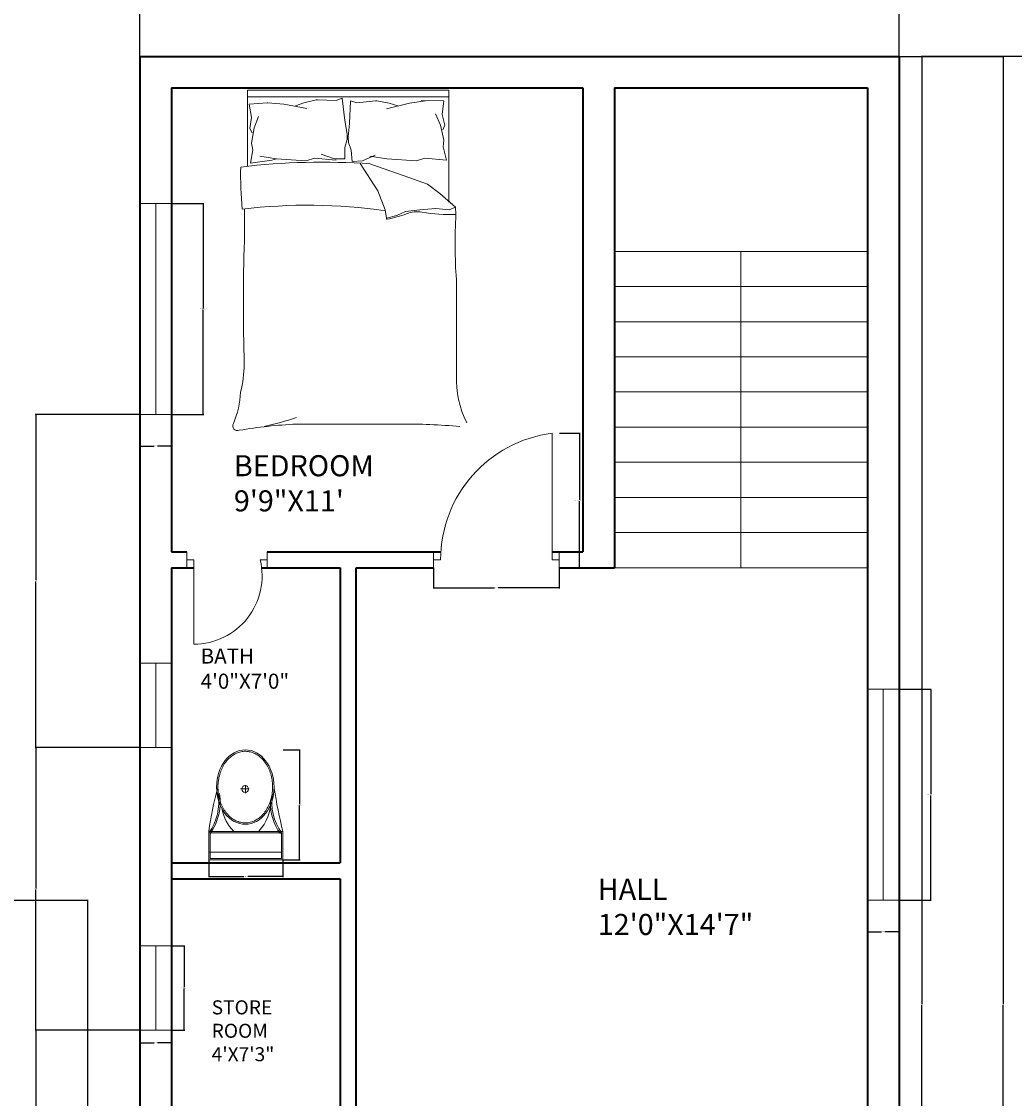
# Model space of a CAD drawing. Units: inches. Extents: x 2003 to 3241, y 1726 to 2849.
# Tile 4 of 7: x 2317 to 2599, y 2073 to 2380. Entities that reach past the tile are written whole.
import ezdxf

# ---------------------------------------------------------------- set-up
doc = ezdxf.new("R2010")
doc.units = ezdxf.units.IN
for name, color, linetype, lineweight in [('A-ANNO-DIMS', 2, 'Continuous', 18), ('A-AREA-IDEN', 7, 'Continuous', 18), ('A-DOOR', 3, 'Continuous', 18), ('A-FLOR-FIXT', 9, 'Continuous', 18), ('A-FLOR-STRS', 7, 'Continuous', 18), ('A-FURN', 8, 'Continuous', 13), ('A-GLAZ', 4, 'Continuous', 18), ('A-WALL', 7, 'Continuous', 35)]:
    doc.layers.add(name, color=color, linetype=linetype, lineweight=lineweight)
doc.styles.add('Annotative', font='arial.ttf')
doc.styles.get("Standard").update_dxf_attribs({"font": 'arial.ttf'})
doc.dimstyles.get("Standard").update_dxf_attribs({"dimtxt": 0.18, "dimasz": 0.18, "dimexe": 0.18, "dimexo": 0.0625, "dimgap": 0.09, "dimtad": 0, "dimtih": 1, "dimtoh": 1, "dimdec": 4, "dimzin": 0, "dimdsep": 46, "dimtxsty": 'Standard', "dimcen": 0.09, "dimadec": 0, "dimazin": 0, "dimtfac": 1, "dimtdec": 4, "dimtofl": 0, "dimtmove": 0, "dimatfit": 3, "dimfxl": 1, "dimtolj": 1, "dimtzin": 0, "dimarcsym": 0})

# ---------------------------------------------------------------- blocks, each defined once
blk = doc.blocks.new('A$C31115884')
for p, q in [((283.1, 497.7), (223.4, 497.7)), ((257.5, 466.4), (257.5, 523.2)), ((0, 200), (0, 0)), ((520, 200), (0, 200)), ((10, 190), (10, 10)), ((510, 190), (10, 190)), ((510, 10), (510, 190)), ((520, 0), (520, 200)), ((510, 54.5), (0, 54.5)), ((10, 10), (510, 10)), ((0, 0), (520, 0))]:
    blk.add_line(p, q)
blk.add_circle((255.6, 496.4), 23.6)
for centre, radius, start, end in [((2777.7, -204.6), 2807, 165.4549, 171.71327), ((-294.5, 403.3), 364.7, 324.20913, 9.34987), ((-294.5, 403.3), 374.7, 324.20913, 9.34987), ((805.8, 403.3), 364.7, 170.65013, 215.79087), ((3237, 905), 2807, 188.28673, 194.5451), ((139.5, 406.2), 293.5, 315.84364, 2.65635), ((805.8, 403.3), 374.7, 179.20365, 215.79087), ((383.6, 406.2), 293.5, 190.27735, 224.15636)]:
    blk.add_arc(centre, radius, start, end)
blk.add_ellipse((256.2, 509.9), major_axis=(0, -260.7), ratio=0.772727)
blk.add_open_spline([(256.2, 259.2), (263.1, 259.2), (270, 259.7), (287.8, 262.3), (298.7, 265.1), (319.9, 273.1), (330.2, 278.4), (350.1, 291.1), (359.7, 298.7), (377.7, 315.9), (386.2, 325.5), (401.7, 346.6), (408.8, 358.1), (421.3, 382.5), (426.8, 395.5), (435.9, 422.4), (439.5, 436.4), (444.8, 465.1), (446.5, 479.7), (447.9, 509.2), (447.6, 524), (445, 553.3), (442.7, 567.8), (436.3, 596), (432.1, 609.7), (421.9, 636), (416, 648.6), (402.5, 672.1), (395, 683), (378.6, 703), (369.8, 712.1), (351.1, 728), (341.3, 734.8), (320.9, 746.2), (310.4, 750.7), (288.9, 757.3), (278, 759.4), (256, 761), (245, 760.6), (223.1, 757.2), (212.3, 754.3), (191.1, 746.1), (180.8, 740.7), (160.9, 727.8), (151.4, 720.1), (133.5, 702.7), (125.1, 693), (109.6, 671.7), (102.6, 660.2), (90.2, 635.7), (84.9, 622.7), (76, 595.6), (72.4, 581.6), (67.2, 552.9), (65.6, 538.2), (64.4, 508.8), (64.8, 494), (67.5, 464.7), (69.9, 450.2), (76.6, 422), (80.8, 408.3), (91.1, 382.2), (97.2, 369.7), (110.8, 346.3), (118.4, 335.4), (134.8, 315.6), (143.7, 306.7), (162.4, 290.9), (172.3, 284.2), (192.8, 273), (203.3, 268.6), (224.8, 262.2), (235.8, 260.2), (249.9, 259.3), (253, 259.2), (256.2, 259.2)], degree=3, knots=[0, 0, 0, 0, 0.110105, 0.110105, 0.285049, 0.285049, 0.459994, 0.459994, 0.634938, 0.634938, 0.809882, 0.809882, 0.984827, 0.984827, 1.159771, 1.159771, 1.334715, 1.334715, 1.50966, 1.50966, 1.684604, 1.684604, 1.859549, 1.859549, 2.034493, 2.034493, 2.209437, 2.209437, 2.384382, 2.384382, 2.559326, 2.559326, 2.73427, 2.73427, 2.909215, 2.909215, 3.084159, 3.084159, 3.259103, 3.259103, 3.434048, 3.434048, 3.608992, 3.608992, 3.783936, 3.783936, 3.958881, 3.958881, 4.133825, 4.133825, 4.30877, 4.30877, 4.483714, 4.483714, 4.658658, 4.658658, 4.833603, 4.833603, 5.008547, 5.008547, 5.183491, 5.183491, 5.358436, 5.358436, 5.53338, 5.53338, 5.708324, 5.708324, 5.883269, 5.883269, 6.058213, 6.058213, 6.233158, 6.233158, 6.283185, 6.283185, 6.283185, 6.283185])
blk = doc.blocks.new('WIN-60-1')
for p, q in [((0, 60), (9, 60)), ((9, 60), (4.5, 60)), ((4.5, 60), (4.5, 0)), ((4.5, 0), (0, 0)), ((0, 0), (9, 0))]:
    blk.add_line(p, q)
blk = doc.blocks.new('WIN-60-2')
for p, q in [((9, 60), (0, 60)), ((0, 60), (4.5, 60)), ((4.5, 60), (4.5, 0)), ((4.5, 0), (0, 0)), ((0, 0), (9, 0))]:
    blk.add_line(p, q)
blk = doc.blocks.new('WIN-24-1')
for p, q in [((0, 24), (9, 24)), ((9, 24), (4.5, 24)), ((4.5, 24), (4.5, 0)), ((4.5, 0), (0, 0)), ((0, 0), (9, 0))]:
    blk.add_line(p, q)
blk = doc.blocks.new('WIN-24-2')
for p, q in [((0, 24), (9, 24)), ((9, 24), (4.5, 24)), ((4.5, 24), (4.5, 0)), ((9, 0), (0, 0)), ((4.5, 0), (9, 0))]:
    blk.add_line(p, q)
blk = doc.blocks.new('DOOR-BEDROOM-UPPER')
for p, q in [((33.76, 2.25), (33.76, 38.25)), ((0, 4.5), (0, 0)), ((35.76, 4.5), (35.76, 0)), ((0, 0), (0, 2.25)), ((0, 2.25), (2, 2.25)), ((35.76, 2.25), (33.76, 2.25)), ((35.76, 0), (35.76, 2.25))]:
    blk.add_line(p, q)
blk.add_arc((38.28, 2.25), 36.28, 97.1626, 180)
blk = doc.blocks.new('STAIR-UPPER-RUN')
for p, q in [((0, 90), (72, 90)), ((36, 0), (36, 90)), ((72, 90), (36, 90)), ((0, 80), (72, 80)), ((72, 80), (36, 80)), ((0, 70), (72, 70)), ((72, 70), (36, 70)), ((0, 60), (72, 60)), ((72, 60), (36, 60)), ((0, 50), (72, 50)), ((72, 50), (36, 50)), ((0, 40), (72, 40)), ((72, 40), (36, 40)), ((0, 30), (72, 30)), ((72, 30), (36, 30)), ((0, 20), (72, 20)), ((72, 20), (36, 20)), ((0, 10), (72, 10)), ((72, 10), (36, 10)), ((0, 0), (72, 0)), ((72, 0), (36, 0))]:
    blk.add_line(p, q)
blk = doc.blocks.new('BED-DOUBLE')
for p, q in [((4.17, 75.16), (4.17, 96.87)), ((4.17, 96.87), (61.46, 96.87)), ((4.17, 95.03), (61.46, 95.03)), ((61.46, 96.87), (61.46, 64.97)), ((4.67, 92.87), (9.81, 93.27)), ((4.67, 92.9), (5.36, 89.08)), ((9.81, 93.27), (9.93, 93.24)), ((9.93, 93.24), (14.52, 92.9)), ((14.52, 92.9), (21.1, 91.68)), ((17.81, 92.38), (20.24, 93.24)), ((20.24, 93.24), (23.7, 94.11)), ((23.7, 94.11), (24.09, 94.11)), ((24.09, 94.11), (29.42, 93.94)), ((29.42, 93.94), (31.15, 94.63)), ((31.15, 94.63), (31.84, 88.22)), ((33.54, 93.89), (33.25, 87.44)), ((35.31, 93.3), (33.54, 93.89)), ((40.62, 93.81), (35.31, 93.3)), ((41.01, 93.83), (40.62, 93.81)), ((44.52, 93.18), (41.01, 93.83)), ((50.25, 93.19), (43.75, 91.57)), ((47, 92.47), (44.52, 93.18)), ((54.8, 93.82), (50.25, 93.19)), ((60.08, 93.81), (53.6, 93.92)), ((53.6, 93.92), (54.8, 93.82)), ((60.08, 93.81), (59.62, 89.96)), ((5.36, 89.08), (4.84, 85.96)), ((6.06, 86.14), (7.27, 89.43)), ((59.12, 86.97), (57.7, 90.18)), ((59.62, 89.96), (60.34, 86.88)), ((4.84, 85.96), (5.54, 84.75)), ((5.36, 81.8), (6.06, 86.14)), ((31.84, 88.22), (32.54, 84.4)), ((33.25, 87.44), (32.79, 83.59)), ((60.08, 82.69), (59.12, 86.97)), ((60.34, 86.88), (59.72, 85.62)), ((32.54, 82.84), (31.84, 80.59)), ((32.54, 84.4), (32.54, 82.84)), ((32.79, 83.59), (32.89, 82.03)), ((5.02, 76.08), (5.71, 79.9)), ((5.71, 79.9), (5.36, 81.8)), ((31.84, 80.59), (31.84, 77.38)), ((32.89, 82.03), (33.72, 79.83)), ((33.72, 79.83), (33.93, 76.62)), ((59.85, 80.77), (60.08, 82.69)), ((60.78, 77), (59.85, 80.77)), ((11.13, 76.95), (5.02, 76.08)), ((7.65, 78.14), (12.48, 77.34)), ((12.48, 77.34), (11.13, 76.95)), ((12.48, 77.34), (20.89, 76.82)), ((20.89, 76.82), (23.24, 77.49)), ((23.24, 77.49), (29.39, 77)), ((28.9, 77.38), (25.13, 78.68)), ((31.84, 77.38), (28.9, 77.38)), ((33.93, 76.62), (36.87, 76.8)), ((36.87, 76.8), (40.55, 78.34)), ((39.04, 78.14), (43.87, 77.34)), ((43.87, 77.34), (52.28, 76.82)), ((52.28, 76.82), (54.63, 77.49)), ((54.63, 77.49), (60.78, 77)), ((36.28, 76.03), (41.3, 68.25)), ((48.73, 72.52), (38.73, 76.03)), ((55.41, 70.1), (48.73, 72.52)), ((41.3, 68.25), (43.34, 62.87)), ((58.94, 67.51), (55.41, 70.1)), ((63.38, 63.61), (58.94, 67.51)), ((43.34, 62.87), (43.71, 60.45)), ((46.68, 61.2), (49.1, 62.31)), ((49.1, 62.31), (53.18, 62.87)), ((53.18, 62.87), (57.82, 63.24)), ((57.82, 63.24), (61.54, 62.87)), ((61.54, 62.87), (63.38, 63.61)), ((63.48, 61.52), (63.38, 63.61, 4.64)), ((43.71, 60.45), (46.68, 61.2)), ((18.06, 1.87), (47.57, 1.87))]:
    blk.add_line(p, q)
for centre, radius, start, end in [((102.1, 72.78), 99.87, 178.7218, 185.604), ((25.61, -121.38), 197.77, 86.0865, 96.7821), ((21.29, -90.53), 154.68, 81.7845, 96.9006), ((-200.58, 59.5), 203.94, 358.4762, 1.0082), ((37.35, 95.1), 35.55, 280.6617, 289.8806), ((52.44, 54.83), 7.46, 78.6608, 113.7384), ((61.53, 104.85), 43.38, 259.8763, 272.5657), ((218.51, 53.34), 155.25, 176.9791, 183.8365), ((43.92, 60.38), 0.221, 160.2464, 271.1377), ((581.23, 36.19), 578.22, 178.22771, 181.71854), ((-5405.34, 15.56), 5469.02, 0.00217, 0.28689), ((-32.25, 19.53), 35.53, 346.0648, 358.9113), ((91.3, 14.55), 27.65, 177.4714, 206.4681), ((-25.97, 12.62), 28.25, 337.9751, 356.652), ((-20.65, 125.3), 127.63, 283.3832, 287.7053), ((1.3, 1.3), 1.31, 146.1736, 293.4781), ((25.69, -143.9), 145.97, 92.9958, 99.4091), ((49.34, -157.62), 159.5, 84.4998, 90.6351)]:
    blk.add_arc(centre, radius, start, end)
blk = doc.blocks.new('*D22')
at = {"layer": 'A-ANNO-DIMS', "color": 0, "lineweight": -2, "transparency": 16777216}
for p, q in [((2359.36, 2328.01), (2368.48, 2328.01)), ((2368.3, 2327.83), (2368.3, 2298.2)), ((2368.3, 2268.19), (2368.3, 2297.83)), ((2359.36, 2268.01), (2368.48, 2268.01))]:
    blk.add_line(p, q, dxfattribs=at)
at = {"layer": 'A-ANNO-DIMS', "color": 0, "transparency": 16777216}
for points in [[(2368.27, 2327.83), (2368.33, 2327.83), (2368.3, 2328.01)], [(2368.27, 2268.19), (2368.33, 2268.19), (2368.3, 2268.01)]]:
    blk.add_solid(points, dxfattribs=at)
at = {"layer": 'Defpoints', "color": 0, "transparency": 16777216}
for p in [(2359.3, 2328.01), (2368.3, 2328.01), (2359.3, 2268.01)]:
    blk.add_point(p, dxfattribs=at)
at = {"layer": 'A-ANNO-DIMS', "color": 0, "transparency": 16777216, "insert": (2368.3, 2298.01), "char_height": 0.18, "attachment_point": 5}
blk.add_mtext('\\A1;WINDOW 60 TYP.', dxfattribs=at)
blk = doc.blocks.new('*D23')
at = {"layer": 'A-ANNO-DIMS', "color": 0, "lineweight": -2, "transparency": 16777216}
for p, q in [((2350.3, 2267.95), (2350.3, 2258.83)), ((2359.3, 2267.95), (2359.3, 2258.83)), ((2350.48, 2259.01), (2354.34, 2259.01)), ((2359.12, 2259.01), (2355.26, 2259.01))]:
    blk.add_line(p, q, dxfattribs=at)
at = {"layer": 'A-ANNO-DIMS', "color": 0, "transparency": 16777216}
for points in [[(2350.48, 2259.04), (2350.48, 2258.98), (2350.3, 2259.01)], [(2359.12, 2259.04), (2359.12, 2258.98), (2359.3, 2259.01)]]:
    blk.add_solid(points, dxfattribs=at)
at = {"layer": 'Defpoints', "color": 0, "transparency": 16777216}
for p in [(2350.3, 2268.01), (2359.3, 2268.01), (2359.3, 2259.01)]:
    blk.add_point(p, dxfattribs=at)
at = {"layer": 'A-ANNO-DIMS', "color": 0, "transparency": 16777216, "insert": (2354.8, 2259.01), "char_height": 0.18, "attachment_point": 5}
blk.add_mtext('\\A1;9 TYP.', dxfattribs=at)
blk = doc.blocks.new('*D28')
at = {"layer": 'A-ANNO-DIMS', "color": 0, "lineweight": -2, "transparency": 16777216}
for p, q in [((2391.06, 2172.57), (2395.87, 2172.57)), ((2395.69, 2172.39), (2395.69, 2157.1)), ((2395.69, 2141.44), (2395.69, 2156.73)), ((2391.06, 2141.26), (2395.87, 2141.26))]:
    blk.add_line(p, q, dxfattribs=at)
at = {"layer": 'A-ANNO-DIMS', "color": 0, "transparency": 16777216}
for points in [[(2395.66, 2172.39), (2395.72, 2172.39), (2395.69, 2172.57)], [(2395.66, 2141.44), (2395.72, 2141.44), (2395.69, 2141.26)]]:
    blk.add_solid(points, dxfattribs=at)
at = {"layer": 'Defpoints', "color": 0, "transparency": 16777216}
for p in [(2391, 2172.57), (2395.69, 2172.57), (2391, 2141.26)]:
    blk.add_point(p, dxfattribs=at)
at = {"layer": 'A-ANNO-DIMS', "color": 0, "transparency": 16777216, "insert": (2395.69, 2156.92), "char_height": 0.18, "attachment_point": 5}
blk.add_mtext('\\A1;WC 31 TYP.', dxfattribs=at)
blk = doc.blocks.new('*D29')
at = {"layer": 'A-ANNO-DIMS', "color": 0, "lineweight": -2, "transparency": 16777216}
for p, q in [((2369.87, 2141.2), (2369.87, 2136.39)), ((2391, 2141.2), (2391, 2136.39)), ((2370.05, 2136.57), (2379.91, 2136.57)), ((2390.82, 2136.57), (2380.97, 2136.57))]:
    blk.add_line(p, q, dxfattribs=at)
at = {"layer": 'A-ANNO-DIMS', "color": 0, "transparency": 16777216}
for points in [[(2370.05, 2136.6), (2370.05, 2136.54), (2369.87, 2136.57)], [(2390.82, 2136.6), (2390.82, 2136.54), (2391, 2136.57)]]:
    blk.add_solid(points, dxfattribs=at)
at = {"layer": 'Defpoints', "color": 0, "transparency": 16777216}
for p in [(2369.87, 2141.26), (2391, 2141.26), (2391, 2136.57)]:
    blk.add_point(p, dxfattribs=at)
at = {"layer": 'A-ANNO-DIMS', "color": 0, "transparency": 16777216, "insert": (2380.44, 2136.57), "char_height": 0.18, "attachment_point": 5}
blk.add_mtext('\\A1;21 TYP.', dxfattribs=at)
blk = doc.blocks.new('*D30')
at = {"layer": 'A-ANNO-DIMS', "color": 0, "lineweight": -2, "transparency": 16777216}
for p, q in [((2566.36, 2189.81), (2575.48, 2189.81)), ((2575.3, 2189.63), (2575.3, 2160)), ((2575.3, 2129.99), (2575.3, 2159.63)), ((2566.36, 2129.81), (2575.48, 2129.81))]:
    blk.add_line(p, q, dxfattribs=at)
at = {"layer": 'A-ANNO-DIMS', "color": 0, "transparency": 16777216}
for points in [[(2575.27, 2189.63), (2575.33, 2189.63), (2575.3, 2189.81)], [(2575.27, 2129.99), (2575.33, 2129.99), (2575.3, 2129.81)]]:
    blk.add_solid(points, dxfattribs=at)
at = {"layer": 'Defpoints', "color": 0, "transparency": 16777216}
for p in [(2566.3, 2189.81), (2575.3, 2189.81), (2566.3, 2129.81)]:
    blk.add_point(p, dxfattribs=at)
at = {"layer": 'A-ANNO-DIMS', "color": 0, "transparency": 16777216, "insert": (2575.3, 2159.81), "char_height": 0.18, "attachment_point": 5}
blk.add_mtext('\\A1;WINDOW 60 TYP.', dxfattribs=at)
blk = doc.blocks.new('*D31')
at = {"layer": 'A-ANNO-DIMS', "color": 0, "lineweight": -2, "transparency": 16777216}
for p, q in [((2557.3, 2129.75), (2557.3, 2120.63)), ((2566.3, 2129.75), (2566.3, 2120.63)), ((2557.48, 2120.81), (2561.34, 2120.81)), ((2566.12, 2120.81), (2562.26, 2120.81))]:
    blk.add_line(p, q, dxfattribs=at)
at = {"layer": 'A-ANNO-DIMS', "color": 0, "transparency": 16777216}
for points in [[(2557.48, 2120.84), (2557.48, 2120.78), (2557.3, 2120.81)], [(2566.12, 2120.84), (2566.12, 2120.78), (2566.3, 2120.81)]]:
    blk.add_solid(points, dxfattribs=at)
at = {"layer": 'Defpoints', "color": 0, "transparency": 16777216}
for p in [(2557.3, 2129.81), (2566.3, 2129.81), (2566.3, 2120.81)]:
    blk.add_point(p, dxfattribs=at)
at = {"layer": 'A-ANNO-DIMS', "color": 0, "transparency": 16777216, "insert": (2561.8, 2120.81), "char_height": 0.18, "attachment_point": 5}
blk.add_mtext('\\A1;9 TYP.', dxfattribs=at)
blk = doc.blocks.new('*D32')
at = {"layer": 'A-ANNO-DIMS', "color": 0, "lineweight": -2, "transparency": 16777216}
for p, q in [((2359.36, 2116.82), (2363.08, 2116.82)), ((2362.9, 2116.64), (2362.9, 2105.01)), ((2362.9, 2093), (2362.9, 2104.64)), ((2359.36, 2092.82), (2363.08, 2092.82))]:
    blk.add_line(p, q, dxfattribs=at)
at = {"layer": 'A-ANNO-DIMS', "color": 0, "transparency": 16777216}
for points in [[(2362.87, 2116.64), (2362.93, 2116.64), (2362.9, 2116.82)], [(2362.87, 2093), (2362.93, 2093), (2362.9, 2092.82)]]:
    blk.add_solid(points, dxfattribs=at)
at = {"layer": 'Defpoints', "color": 0, "transparency": 16777216}
for p in [(2359.3, 2116.82), (2362.9, 2116.82), (2359.3, 2092.82)]:
    blk.add_point(p, dxfattribs=at)
at = {"layer": 'A-ANNO-DIMS', "color": 0, "transparency": 16777216, "insert": (2362.9, 2104.82), "char_height": 0.18, "attachment_point": 5}
blk.add_mtext('\\A1;WINDOW 24 TYP.', dxfattribs=at)
blk = doc.blocks.new('*D33')
at = {"layer": 'A-ANNO-DIMS', "color": 0, "lineweight": -2, "transparency": 16777216}
for p, q in [((2350.3, 2092.76), (2350.3, 2089.04)), ((2359.3, 2092.76), (2359.3, 2089.04)), ((2350.48, 2089.22), (2354.34, 2089.22)), ((2359.12, 2089.22), (2355.26, 2089.22))]:
    blk.add_line(p, q, dxfattribs=at)
at = {"layer": 'A-ANNO-DIMS', "color": 0, "transparency": 16777216}
for points in [[(2350.48, 2089.25), (2350.48, 2089.19), (2350.3, 2089.22)], [(2359.12, 2089.25), (2359.12, 2089.19), (2359.3, 2089.22)]]:
    blk.add_solid(points, dxfattribs=at)
at = {"layer": 'Defpoints', "color": 0, "transparency": 16777216}
for p in [(2350.3, 2092.82), (2359.3, 2092.82), (2359.3, 2089.22)]:
    blk.add_point(p, dxfattribs=at)
at = {"layer": 'A-ANNO-DIMS', "color": 0, "transparency": 16777216, "insert": (2354.8, 2089.22), "char_height": 0.18, "attachment_point": 5}
blk.add_mtext('\\A1;9 TYP.', dxfattribs=at)
blk = doc.blocks.new('*D46')
at = {"layer": 'A-ANNO-DIMS', "color": 0, "lineweight": -2, "transparency": 16777216}
for p, q in [((2469.68, 2262.66), (2475.53, 2262.66)), ((2475.35, 2262.48), (2475.35, 2243.72)), ((2475.35, 2224.59), (2475.35, 2243.36)), ((2469.68, 2224.41), (2475.53, 2224.41))]:
    blk.add_line(p, q, dxfattribs=at)
at = {"layer": 'A-ANNO-DIMS', "color": 0, "transparency": 16777216}
for points in [[(2475.32, 2262.48), (2475.38, 2262.48), (2475.35, 2262.66)], [(2475.32, 2224.59), (2475.38, 2224.59), (2475.35, 2224.41)]]:
    blk.add_solid(points, dxfattribs=at)
at = {"layer": 'Defpoints', "color": 0, "transparency": 16777216}
for p in [(2469.62, 2262.66), (2475.35, 2262.66), (2469.62, 2224.41)]:
    blk.add_point(p, dxfattribs=at)
at = {"layer": 'A-ANNO-DIMS', "color": 0, "transparency": 16777216, "insert": (2475.35, 2243.54), "char_height": 0.18, "attachment_point": 5}
blk.add_mtext('\\A1;BEDROOM DOOR 38 TYP.', dxfattribs=at)
blk = doc.blocks.new('*D47')
at = {"layer": 'A-ANNO-DIMS', "color": 0, "lineweight": -2, "transparency": 16777216}
for p, q in [((2433.86, 2224.35), (2433.86, 2218.5)), ((2469.62, 2224.35), (2469.62, 2218.5)), ((2434.04, 2218.68), (2451.21, 2218.68)), ((2469.44, 2218.68), (2452.27, 2218.68))]:
    blk.add_line(p, q, dxfattribs=at)
at = {"layer": 'A-ANNO-DIMS', "color": 0, "transparency": 16777216}
for points in [[(2434.04, 2218.71), (2434.04, 2218.65), (2433.86, 2218.68)], [(2469.44, 2218.71), (2469.44, 2218.65), (2469.62, 2218.68)]]:
    blk.add_solid(points, dxfattribs=at)
at = {"layer": 'Defpoints', "color": 0, "transparency": 16777216}
for p in [(2433.86, 2224.41), (2469.62, 2224.41), (2469.62, 2218.68)]:
    blk.add_point(p, dxfattribs=at)
at = {"layer": 'A-ANNO-DIMS', "color": 0, "transparency": 16777216, "insert": (2451.74, 2218.68), "char_height": 0.18, "attachment_point": 5}
blk.add_mtext('\\A1;36 TYP.', dxfattribs=at)
blk = doc.blocks.new('*D67')
at = {"layer": 'A-ANNO-DIMS', "color": 0, "lineweight": -2, "transparency": 16777216}
for p, q in [((2305.84, 2129.81), (2335.61, 2129.81)), ((2335.43, 2129.63), (2335.43, 2026.55)), ((2335.43, 1923.09), (2335.43, 2026.18)), ((2305.84, 1922.91), (2335.61, 1922.91))]:
    blk.add_line(p, q, dxfattribs=at)
at = {"layer": 'A-ANNO-DIMS', "color": 0, "transparency": 16777216}
for points in [[(2335.4, 2129.63), (2335.46, 2129.63), (2335.43, 2129.81)], [(2335.4, 1923.09), (2335.46, 1923.09), (2335.43, 1922.91)]]:
    blk.add_solid(points, dxfattribs=at)
at = {"layer": 'Defpoints', "color": 0, "transparency": 16777216}
for p in [(2305.78, 2129.81), (2335.43, 2129.81), (2305.78, 1922.91)]:
    blk.add_point(p, dxfattribs=at)
at = {"layer": 'A-ANNO-DIMS', "color": 0, "transparency": 16777216, "insert": (2335.43, 2026.36), "char_height": 0.18, "attachment_point": 5}
blk.add_mtext('\\A1;206.9', dxfattribs=at)
blk = doc.blocks.new('*D70')
at = {"layer": 'A-ANNO-DIMS', "color": 0, "lineweight": -2, "transparency": 16777216}
for p, q in [((2350.3, 2369.98), (2350.3, 2399.74)), ((2350.48, 2399.56), (2458.01, 2399.56)), ((2566.12, 2399.56), (2458.59, 2399.56)), ((2566.3, 2369.98), (2566.3, 2399.74))]:
    blk.add_line(p, q, dxfattribs=at)
at = {"layer": 'A-ANNO-DIMS', "color": 0, "transparency": 16777216}
for points in [[(2350.48, 2399.59), (2350.48, 2399.53), (2350.3, 2399.56)], [(2566.12, 2399.59), (2566.12, 2399.53), (2566.3, 2399.56)]]:
    blk.add_solid(points, dxfattribs=at)
at = {"layer": 'Defpoints', "color": 0, "transparency": 16777216}
for p in [(2566.3, 2399.56), (2350.3, 2369.91), (2566.3, 2369.91)]:
    blk.add_point(p, dxfattribs=at)
at = {"layer": 'A-ANNO-DIMS', "color": 0, "transparency": 16777216, "insert": (2458.3, 2399.56), "char_height": 0.18, "attachment_point": 5}
blk.add_mtext('\\A1;216', dxfattribs=at)
blk = doc.blocks.new('*D71')
at = {"layer": 'A-ANNO-DIMS', "color": 0, "lineweight": -2, "transparency": 16777216}
for p, q in [((2566.36, 2369.91), (2596.13, 2369.91)), ((2595.95, 2369.73), (2595.95, 2100.35)), ((2595.95, 1830.59), (2595.95, 2099.98)), ((2566.36, 1830.41), (2596.13, 1830.41))]:
    blk.add_line(p, q, dxfattribs=at)
at = {"layer": 'A-ANNO-DIMS', "color": 0, "transparency": 16777216}
for points in [[(2595.92, 2369.73), (2595.98, 2369.73), (2595.95, 2369.91)], [(2595.92, 1830.59), (2595.98, 1830.59), (2595.95, 1830.41)]]:
    blk.add_solid(points, dxfattribs=at)
at = {"layer": 'Defpoints', "color": 0, "transparency": 16777216}
for p in [(2566.3, 2369.91), (2595.95, 2369.91), (2566.3, 1830.41)]:
    blk.add_point(p, dxfattribs=at)
at = {"layer": 'A-ANNO-DIMS', "color": 0, "transparency": 16777216, "insert": (2595.95, 2100.16), "char_height": 0.18, "attachment_point": 5}
blk.add_mtext('\\A1;539.5', dxfattribs=at)
blk = doc.blocks.new('*D73')
at = {"layer": 'A-ANNO-DIMS', "color": 0, "lineweight": -2, "transparency": 16777216}
for p, q in [((2350.24, 2092.82), (2320.47, 2092.82)), ((2320.65, 2092.64), (2320.65, 2022.3)), ((2320.65, 1951.6), (2320.65, 2021.94)), ((2350.24, 1951.42), (2320.47, 1951.42))]:
    blk.add_line(p, q, dxfattribs=at)
at = {"layer": 'A-ANNO-DIMS', "color": 0, "transparency": 16777216}
for points in [[(2320.62, 2092.64), (2320.68, 2092.64), (2320.65, 2092.82)], [(2320.62, 1951.6), (2320.68, 1951.6), (2320.65, 1951.42)]]:
    blk.add_solid(points, dxfattribs=at)
at = {"layer": 'Defpoints', "color": 0, "transparency": 16777216}
for p in [(2320.65, 2092.82), (2350.3, 2092.82), (2350.3, 1951.42)]:
    blk.add_point(p, dxfattribs=at)
at = {"layer": 'A-ANNO-DIMS', "color": 0, "transparency": 16777216, "insert": (2320.65, 2022.12), "char_height": 0.18, "attachment_point": 5}
blk.add_mtext('\\A1;141.4', dxfattribs=at)
blk = doc.blocks.new('*D74')
at = {"layer": 'A-ANNO-DIMS', "color": 0, "lineweight": -2, "transparency": 16777216}
for p, q in [((2350.24, 2173.28), (2320.47, 2173.28)), ((2320.65, 2173.1), (2320.65, 2133.23)), ((2320.65, 2093), (2320.65, 2132.87)), ((2350.24, 2092.82), (2320.47, 2092.82))]:
    blk.add_line(p, q, dxfattribs=at)
at = {"layer": 'A-ANNO-DIMS', "color": 0, "transparency": 16777216}
for points in [[(2320.62, 2173.1), (2320.68, 2173.1), (2320.65, 2173.28)], [(2320.62, 2093), (2320.68, 2093), (2320.65, 2092.82)]]:
    blk.add_solid(points, dxfattribs=at)
at = {"layer": 'Defpoints', "color": 0, "transparency": 16777216}
for p in [(2320.65, 2173.28), (2350.3, 2173.28), (2350.3, 2092.82)]:
    blk.add_point(p, dxfattribs=at)
at = {"layer": 'A-ANNO-DIMS', "color": 0, "transparency": 16777216, "insert": (2320.65, 2133.05), "char_height": 0.18, "attachment_point": 5}
blk.add_mtext('\\A1;80.46', dxfattribs=at)
blk = doc.blocks.new('*D75')
at = {"layer": 'A-ANNO-DIMS', "color": 0, "lineweight": -2, "transparency": 16777216}
for p, q in [((2350.24, 2268.01), (2320.47, 2268.01)), ((2320.65, 2267.83), (2320.65, 2220.83)), ((2320.65, 2173.46), (2320.65, 2220.46)), ((2350.24, 2173.28), (2320.47, 2173.28))]:
    blk.add_line(p, q, dxfattribs=at)
at = {"layer": 'A-ANNO-DIMS', "color": 0, "transparency": 16777216}
for points in [[(2320.62, 2267.83), (2320.68, 2267.83), (2320.65, 2268.01)], [(2320.62, 2173.46), (2320.68, 2173.46), (2320.65, 2173.28)]]:
    blk.add_solid(points, dxfattribs=at)
at = {"layer": 'Defpoints', "color": 0, "transparency": 16777216}
for p in [(2320.65, 2268.01), (2350.3, 2268.01), (2350.3, 2173.28)]:
    blk.add_point(p, dxfattribs=at)
at = {"layer": 'A-ANNO-DIMS', "color": 0, "transparency": 16777216, "insert": (2320.65, 2220.65), "char_height": 0.18, "attachment_point": 5}
blk.add_mtext('\\A1;94.73', dxfattribs=at)
blk = doc.blocks.new('*D77')
at = {"layer": 'A-ANNO-DIMS', "color": 0, "lineweight": -2, "transparency": 16777216}
for p, q in [((2632.38, 2369.91), (2572.63, 2369.91)), ((2572.81, 2369.73), (2572.81, 2100.35)), ((2572.81, 1830.59), (2572.81, 2099.98)), ((2632.38, 1830.41), (2572.63, 1830.41))]:
    blk.add_line(p, q, dxfattribs=at)
at = {"layer": 'A-ANNO-DIMS', "color": 0, "transparency": 16777216}
for points in [[(2572.78, 2369.73), (2572.84, 2369.73), (2572.81, 2369.91)], [(2572.78, 1830.59), (2572.84, 1830.59), (2572.81, 1830.41)]]:
    blk.add_solid(points, dxfattribs=at)
at = {"layer": 'Defpoints', "color": 0, "transparency": 16777216}
for p in [(2572.81, 2369.91), (2632.44, 2369.91), (2632.44, 1830.41)]:
    blk.add_point(p, dxfattribs=at)
at = {"layer": 'A-ANNO-DIMS', "color": 0, "transparency": 16777216, "insert": (2572.81, 2100.16), "char_height": 0.18, "attachment_point": 5}
blk.add_mtext('\\A1;539.5', dxfattribs=at)

msp = doc.modelspace()

# ---------------------------------------------------------------- linework, layer by layer
at = {"layer": 'A-DOOR'}
for p, q in [((2363.6497, 2228.9135), (2363.6497, 2224.4135)), ((2386.5194, 2228.9135), (2386.5194, 2224.4135)), ((2363.6497, 2224.4135), (2363.6497, 2226.6635)), ((2363.6497, 2226.6635), (2365.6497, 2226.6635)), ((2365.6497, 2226.6635), (2365.6497, 2202.6635)), ((2386.5194, 2226.6635), (2384.5194, 2226.6635)), ((2386.5194, 2224.4135), (2386.5194, 2226.6635))]:
    msp.add_line(p, q, dxfattribs=at)
msp.add_arc((2365.6497, 2222.0815), 19.418, 270, 13.64856, dxfattribs=at)
at = {"layer": 'A-WALL'}
for p, q in [((2350.3008, 2369.9135), (2566.3008, 2369.9135)), ((2350.3008, 2369.9135), (2350.3008, 1836.4016)), ((2566.3008, 2369.9135), (2566.3008, 1836.4016)), ((2359.3008, 2360.9135), (2359.3008, 2228.9135)), ((2359.3008, 2360.9135), (2476.3008, 2360.9135)), ((2476.3008, 2360.9135), (2476.3008, 2228.9135)), ((2485.3008, 2360.9135), (2485.3008, 2224.4135)), ((2485.3008, 2360.9135), (2557.3008, 2360.9135)), ((2557.3008, 2360.9135), (2557.3008, 2048.9135)), ((2359.3008, 2228.9135), (2363.6497, 2228.9135)), ((2386.5194, 2228.9135), (2435.9278, 2228.9135)), ((2467.6172, 2228.9135), (2476.3008, 2228.9135)), ((2359.3008, 2224.4135), (2365.6497, 2224.4135)), ((2359.3008, 2224.4135), (2359.3008, 1912.4135)), ((2359.3008, 2224.4135), (2365.6497, 2224.4135)), ((2384.9272, 2224.4135), (2407.3008, 2224.4135)), ((2384.9272, 2224.4135), (2407.3008, 2224.4135)), ((2407.3008, 2224.4135), (2407.3008, 2140.4135)), ((2411.8008, 2224.4135), (2433.858, 2224.4135)), ((2411.8008, 2048.9135), (2411.8008, 2224.4135)), ((2469.6172, 2224.4135), (2476.3008, 2224.4135)), ((2476.3008, 2224.4135), (2485.3008, 2224.4135)), ((2359.3008, 2140.4135), (2407.3008, 2140.4135)), ((2359.3008, 2135.9135), (2407.3008, 2135.9135)), ((2407.3008, 2135.9135), (2407.3008, 2048.9135))]:
    msp.add_line(p, q, dxfattribs=at)

# ---------------------------------------------------------------- block references
at = {"layer": 'A-DOOR'}
msp.add_blockref('DOOR-BEDROOM-UPPER', (2433.858, 2224.414), dxfattribs=at)
at = {"layer": 'A-FLOR-FIXT', "xscale": 0.0406268506401408, "yscale": 0.0406268506401408, "zscale": 0.0406268506401408}
msp.add_blockref('A$C31115884', (2369.8725, 2141.2633), dxfattribs=at)
at = {"layer": 'A-FLOR-STRS'}
msp.add_blockref('STAIR-UPPER-RUN', (2485.301, 2224.414), dxfattribs=at)
at = {"layer": 'A-FURN'}
msp.add_blockref('BED-DOUBLE', (2376.7228, 2263.4117), dxfattribs=at)
at = {"layer": 'A-GLAZ'}
for name, p in [('WIN-60-1', (2350.3004, 2268.0124)), ('WIN-24-1', (2350.3004, 2173.279)), ('WIN-60-2', (2557.301, 2129.815)), ('WIN-24-2', (2350.301, 2092.823))]:
    msp.add_blockref(name, p, dxfattribs=at)

# ---------------------------------------------------------------- texts
at = {"layer": 'A-AREA-IDEN', "attachment_point": 1}
for s, width, insert, char_height in [('BEDROOM\\P9\'9"X11\'', 185.10211, (2377.0364, 2256.4294), 6), ('HALL\\P12\'0"X14\'7"', 146.116563, (2480.5703, 2135.8937), 6), ('STORE\\PROOM\\P4\'X7\'3"', 94.761983, (2370.7106, 2101.3034), 4)]:
    msp.add_mtext_dynamic_manual_height_columns(s, width=width, gutter_width=12.5, heights=[0], dxfattribs=dict(at, insert=insert, char_height=char_height))
at = {"layer": 'A-AREA-IDEN', "insert": (2367.587, 2201.4145), "char_height": 4.2927, "width": 96.13195, "attachment_point": 1, "style": 'Annotative'}
msp.add_mtext('BATH\\P4\'0"X7\'0"', dxfattribs=at)

# ---------------------------------------------------------------- dimensions: what is measured, and where the dimension line sits
at = {"layer": 'A-ANNO-DIMS'}
dim = msp.add_linear_dim(base=(2566.3008, 2399.5635), p1=(2350.3008, 2369.9135), p2=(2566.3008, 2369.9135), dimstyle='Standard', override={"dimdec": 0, "dimlfac": 1, "dimrnd": 0, "dimzin": 0, "dimdsep": 46, "dimlunit": 2}, dxfattribs=at)
dim.commit()
dim.dimension.update_dxf_attribs({"geometry": '*D70', "text_midpoint": (2458.3008, 2399.5635)})
for base, p1, p2, override, picture, middle in [((2595.9508, 2369.9135), (2566.3008, 1830.4135), (2566.3008, 2369.9135), {"dimdec": 1, "dimlfac": 1, "dimrnd": 0, "dimzin": 0, "dimdsep": 46, "dimlunit": 2}, '*D71', (2595.9508, 2100.1635)), ((2572.8116, 2369.9135), (2632.4427, 1830.4135), (2632.4427, 2369.9135), {"dimdec": 1, "dimlfac": 1, "dimrnd": 0, "dimzin": 0, "dimdsep": 46, "dimlunit": 2}, '*D77', (2572.8116, 2100.1635)), ((2320.6508, 2268.0126), (2350.3008, 2173.2787), (2350.3008, 2268.0126), {"dimdec": 2, "dimlfac": 1, "dimrnd": 0, "dimzin": 0, "dimdsep": 46, "dimlunit": 2}, '*D75', (2320.6508, 2220.6457)), ((2320.6508, 2173.2787), (2350.3008, 2092.8234), (2350.3008, 2173.2787), {"dimdec": 2, "dimlfac": 1, "dimrnd": 0, "dimzin": 0, "dimdsep": 46, "dimlunit": 2}, '*D74', (2320.6508, 2133.0511)), ((2335.4284, 2129.8149), (2305.7784, 1922.9135), (2305.7784, 2129.8149), {"dimdec": 1, "dimlfac": 1, "dimrnd": 0, "dimzin": 0, "dimdsep": 46, "dimlunit": 2}, '*D67', (2335.4284, 2026.3642)), ((2320.6508, 2092.8234), (2350.3008, 1951.4156), (2350.3008, 2092.8234), {"dimdec": 1, "dimlfac": 1, "dimrnd": 0, "dimzin": 0, "dimdsep": 46, "dimlunit": 2}, '*D73', (2320.6508, 2022.1195))]:
    dim = msp.add_linear_dim(base=base, p1=p1, p2=p2, angle=90, dimstyle='Standard', override=override, dxfattribs=at)
    dim.commit()
    dim.dimension.update_dxf_attribs({"geometry": picture, "text_midpoint": middle})
for base, p1, p2, text, picture, middle in [((2368.3008, 2328.0126), (2359.3008, 2268.0126), (2359.3008, 2328.0126), 'WINDOW <> TYP.', '*D22', (2368.3008, 2298.0126)), ((2475.3547, 2262.6635), (2469.6172, 2224.4135), (2469.6172, 2262.6635), 'BEDROOM DOOR <> TYP.', '*D46', (2475.3547, 2243.5385)), ((2575.3008, 2189.8149), (2566.3008, 2129.8149), (2566.3008, 2189.8149), 'WINDOW <> TYP.', '*D30', (2575.3008, 2159.8149)), ((2395.6943, 2172.5692), (2390.9984, 2141.2633), (2390.9984, 2172.5692), 'WC <> TYP.', '*D28', (2395.6943, 2156.9162)), ((2362.9008, 2116.8234), (2359.3008, 2092.8234), (2359.3008, 2116.8234), 'WINDOW <> TYP.', '*D32', (2362.9008, 2104.8234))]:
    dim = msp.add_linear_dim(base=base, p1=p1, p2=p2, angle=90, text=text, dimstyle='Standard', override={"dimdec": 0, "dimlfac": 1, "dimrnd": 0, "dimzin": 0, "dimdsep": 46, "dimlunit": 2}, dxfattribs=at)
    dim.commit()
    dim.dimension.update_dxf_attribs({"geometry": picture, "text_midpoint": middle})
for base, p1, p2, picture, middle in [((2359.3008, 2259.0126), (2350.3008, 2268.0126), (2359.3008, 2268.0126), '*D23', (2354.8008, 2259.0126)), ((2469.6172, 2218.676), (2433.858, 2224.4135), (2469.6172, 2224.4135), '*D47', (2451.7376, 2218.676)), ((2390.9984, 2136.5675), (2369.8725, 2141.2633), (2390.9984, 2141.2633), '*D29', (2380.4355, 2136.5675)), ((2566.3008, 2120.8149), (2557.3008, 2129.8149), (2566.3008, 2129.8149), '*D31', (2561.8008, 2120.8149)), ((2359.3008, 2089.2234), (2350.3008, 2092.8234), (2359.3008, 2092.8234), '*D33', (2354.8008, 2089.2234))]:
    dim = msp.add_linear_dim(base=base, p1=p1, p2=p2, text='<> TYP.', dimstyle='Standard', override={"dimdec": 0, "dimlfac": 1, "dimrnd": 0, "dimzin": 0, "dimdsep": 46, "dimlunit": 2}, dxfattribs=at)
    dim.commit()
    dim.dimension.update_dxf_attribs({"geometry": picture, "text_midpoint": middle})

doc.saveas('drawing.dxf')
